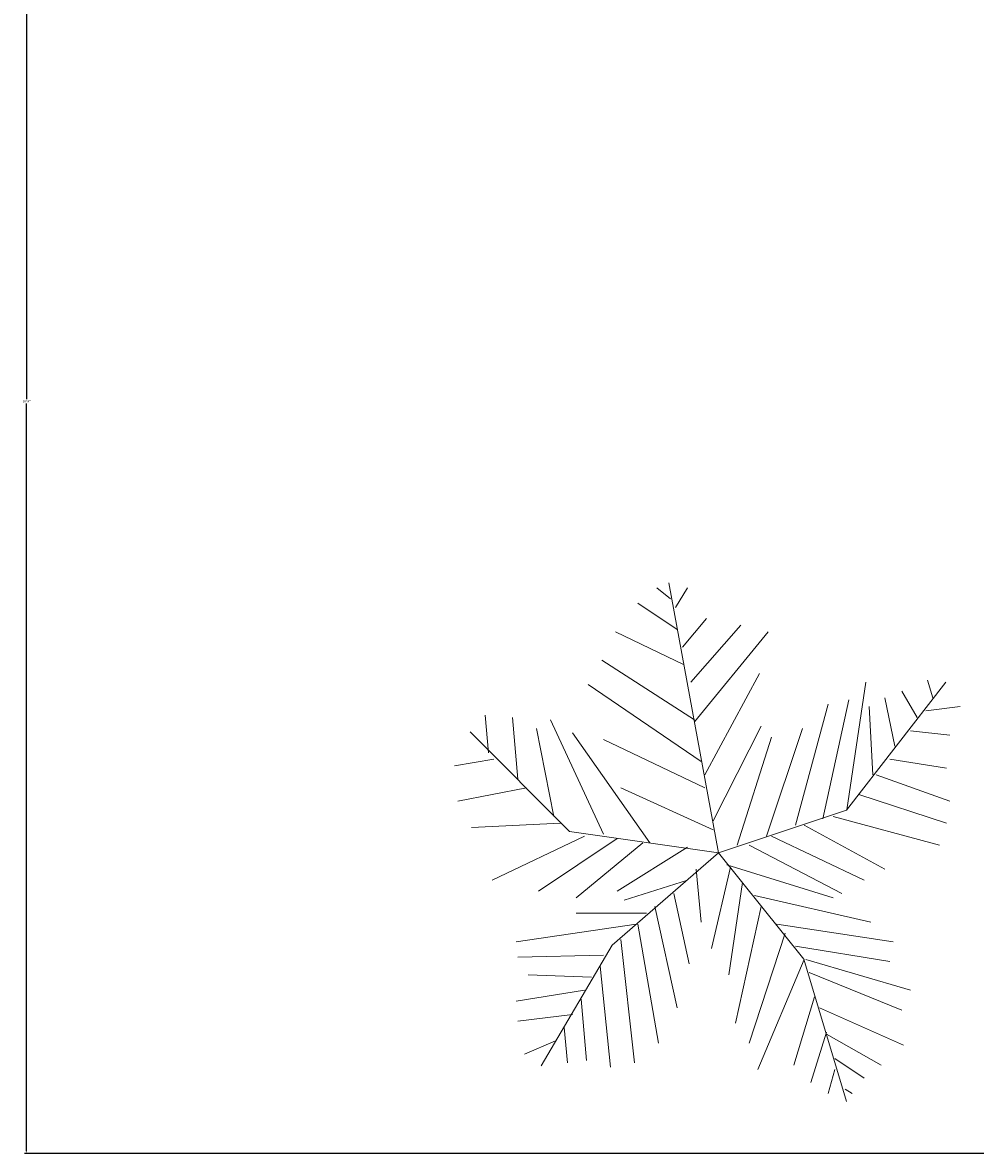
# Model space of a CAD drawing. Units: inches. Extents: x 37 to 824, y -700 to 234.
# Tile 23 of 77: x 78 to 160, y -366 to -269. Entities that reach past the tile are written whole.
import ezdxf

# ---------------------------------------------------------------- set-up
doc = ezdxf.new("R2010")
doc.units = ezdxf.units.IN
doc.header["$MEASUREMENT"] = 0
doc.layers.add('A-ANNO-DIMS', color=2, linetype='Continuous', lineweight=18)
doc.layers.add('A-SITE-PLNT', color=3, linetype='Continuous', lineweight=13)
doc.styles.get("Standard").update_dxf_attribs({"font": 'arial.ttf'})
doc.dimstyles.get("Standard").update_dxf_attribs({"dimtxt": 0.18, "dimasz": 0.18, "dimexe": 0.18, "dimexo": 0.0625, "dimgap": 0.09, "dimtad": 0, "dimtih": 1, "dimtoh": 1, "dimdec": 1, "dimzin": 0, "dimdsep": 46, "dimlunit": 4, "dimtxsty": 'Standard', "dimcen": 0.09, "dimadec": 0, "dimazin": 0, "dimtfac": 1, "dimtdec": 1, "dimtofl": 0, "dimtmove": 0, "dimatfit": 3, "dimfxl": 1, "dimtolj": 1, "dimtzin": 0, "dimarcsym": 0})

# ---------------------------------------------------------------- blocks, each defined once
blk = doc.blocks.new('*U33')
for p, q in [((-10.186, 53.64), (-13.084, 55.962)), ((0, 0), (-10.5, 57)), ((-9.099, 51.782), (-6.563, 55.962)), ((-8.737, 47.138), (-17.069, 52.711)), ((-7.65, 43.423), (-2.578, 49.46)), ((-5.839, 35.992), (4.667, 48.067)), ((-7.288, 39.707), (-21.778, 46.673)), ((-5.114, 27.632), (10.463, 46.673)), ((-5.114, 28.097), (-24.676, 40.636)), ((-2.941, 16.486), (8.652, 37.85)), ((27, 9), (48, 36)), ((27.127, 9.056), (31.112, 35.992)), ((44.153, 36.456), (45.239, 32.741)), ((-3.665, 19.273), (-27.574, 35.527)), ((38.719, 34.134), (41.979, 28.561)), ((16.259, 5.805), (23.142, 31.348)), ((22.055, 7.198), (27.489, 32.277)), ((35.096, 32.741), (37.27, 22.524)), ((-48.585, 21.131), (-49.309, 29.026)), ((31.836, 30.883), (32.561, 16.486)), ((43.791, 29.954), (51.036, 30.883)), ((-43.513, 28.561), (-42.427, 15.558)), ((-35.544, 28.097), (-24.314, 3.947)), ((-1.129, 6.734), (9.014, 26.704)), ((-31.5, 4.5), (-52.5, 25.5)), ((-38.442, 26.239), (-34.819, 7.663)), ((-14.533, 2.09), (-30.834, 25.31)), ((-24.314, 23.917), (-2.941, 13.7)), ((3.942, 1.625), (11.187, 24.381)), ((10.101, 3.483), (17.708, 26.239)), ((40.53, 25.775), (48.862, 24.846)), ((-47.498, 19.737), (-55.83, 18.344)), ((36.183, 19.737), (48.137, 17.88)), ((33.285, 16.486), (48.862, 10.913)), ((-40.615, 13.7), (-55.105, 10.913)), ((-20.691, 13.7), (-1.129, 4.876)), ((29.662, 12.307), (48.137, 6.269)), ((0, 0), (27, 9)), ((24.229, 7.663), (46.688, 1.625)), ((-33.37, 6.269), (-52.207, 5.34)), ((18.07, 5.805), (35.096, -3.483)), ((-28.299, 3.483), (-47.86, -5.805)), ((-21.416, 3.018), (-38.079, -8.128)), ((0, 0), (-31.5, 4.5)), ((11.187, 3.483), (30.749, -5.805)), ((-15.982, 2.09), (-30.11, -9.521)), ((0, 0), (-22.5, -19.5)), ((-6.563, 1.161), (-21.416, -8.128)), ((0, 0), (18, -22.5)), ((6.478, 1.625), (26.04, -8.592)), ((-4.752, -3.483), (-3.665, -14.629)), ((2.493, -3.019), (-1.491, -20.202)), ((1.769, -2.555), (24.229, -9.521)), ((-6.563, -5.805), (-19.967, -9.985)), ((5.029, -6.27), (2.131, -25.775)), ((-9.461, -8.592), (-6.201, -23.453)), ((7.565, -9.056), (32.198, -14.629)), ((-13.446, -11.378), (-8.737, -32.741)), ((9.014, -11.378), (3.58, -35.992)), ((-15.257, -12.772), (-30.11, -12.772)), ((-17.431, -15.094), (-42.789, -18.809)), ((-17.069, -15.094), (-12.721, -40.172)), ((12.274, -15.094), (36.907, -18.809)), ((-20.691, -18.345), (-17.793, -44.352)), ((14.085, -16.951), (6.478, -40.172)), ((-22.5, -19.5), (-37.5, -45)), ((16.259, -19.738), (36.183, -22.989)), ((-24.314, -21.596), (-42.427, -22.06)), ((18.07, -22.524), (8.289, -45.745)), ((18, -22.5), (27, -52.5)), ((18.433, -22.524), (40.53, -29.026)), ((-26.849, -26.24), (-40.253, -25.775)), ((-25.038, -23.918), (-22.865, -45.281)), ((19.157, -25.311), (38.719, -33.206)), ((-28.299, -29.026), (-42.789, -31.348)), ((-29.023, -30.884), (-27.936, -43.887)), ((20.244, -30.419), (15.897, -44.816)), ((21.331, -32.741), (39.081, -40.636)), ((-30.834, -34.135), (-42.427, -35.528)), ((-32.646, -36.921), (-31.921, -44.352)), ((22.78, -37.85), (19.519, -48.532)), ((-34.457, -39.708), (-40.978, -42.494)), ((22.78, -38.314), (34.372, -44.816)), ((24.591, -43.423), (30.749, -47.603)), ((24.591, -45.745), (23.142, -50.854)), ((26.764, -49.925), (28.213, -50.854))]:
    blk.add_line(p, q)
blk = doc.blocks.new('*D59')
at = {"layer": 'A-ANNO-DIMS', "color": 0, "lineweight": -2, "ltscale": 0.5, "transparency": 16777216}
for p, q in [((161.015, -236.91), (78.159, -236.91)), ((78.339, -237.09), (78.339, -301.228)), ((78.339, -365.73), (78.339, -301.591)), ((161.015, -365.91), (78.159, -365.91))]:
    blk.add_line(p, q, dxfattribs=at)
at = {"layer": 'A-ANNO-DIMS', "color": 0, "ltscale": 0.5, "transparency": 16777216}
for points in [[(78.309, -237.09), (78.369, -237.09), (78.339, -236.91)], [(78.309, -365.73), (78.369, -365.73), (78.339, -365.91)]]:
    blk.add_solid(points, dxfattribs=at)
at = {"layer": 'Defpoints', "color": 0, "ltscale": 0.5, "transparency": 16777216}
for p in [(161.077, -236.91), (78.339, -365.91), (161.077, -365.91)]:
    blk.add_point(p, dxfattribs=at)
at = {"layer": 'A-ANNO-DIMS', "color": 0, "ltscale": 0.5, "transparency": 16777216, "insert": (78.339, -301.41), "char_height": 0.18, "attachment_point": 5}
blk.add_mtext('\\A1;10\'-9"', dxfattribs=at)

msp = doc.modelspace()

# ---------------------------------------------------------------- block references
at = {"layer": 'A-SITE-PLNT', "xscale": 0.406169560041474, "yscale": 0.406169560041474, "zscale": 0.406169560041474}
msp.add_blockref('*U33', (137.73, -340.127), dxfattribs=at)

# ---------------------------------------------------------------- dimensions: what is measured, and where the dimension line sits
at = {"layer": 'A-ANNO-DIMS', "ltscale": 0.5}
dim = msp.add_linear_dim(base=(78.339, -365.91), p1=(161.077, -236.91), p2=(161.077, -365.91), angle=90, dimstyle='Standard', override={"dimdec": 1, "dimlfac": 1, "dimrnd": 0, "dimzin": 1, "dimdsep": 46, "dimlunit": 4, "dimfrac": 2}, dxfattribs=at)
dim.commit()
dim.dimension.update_dxf_attribs({"geometry": '*D59', "text_midpoint": (78.339, -301.41)})

doc.saveas('drawing.dxf')
